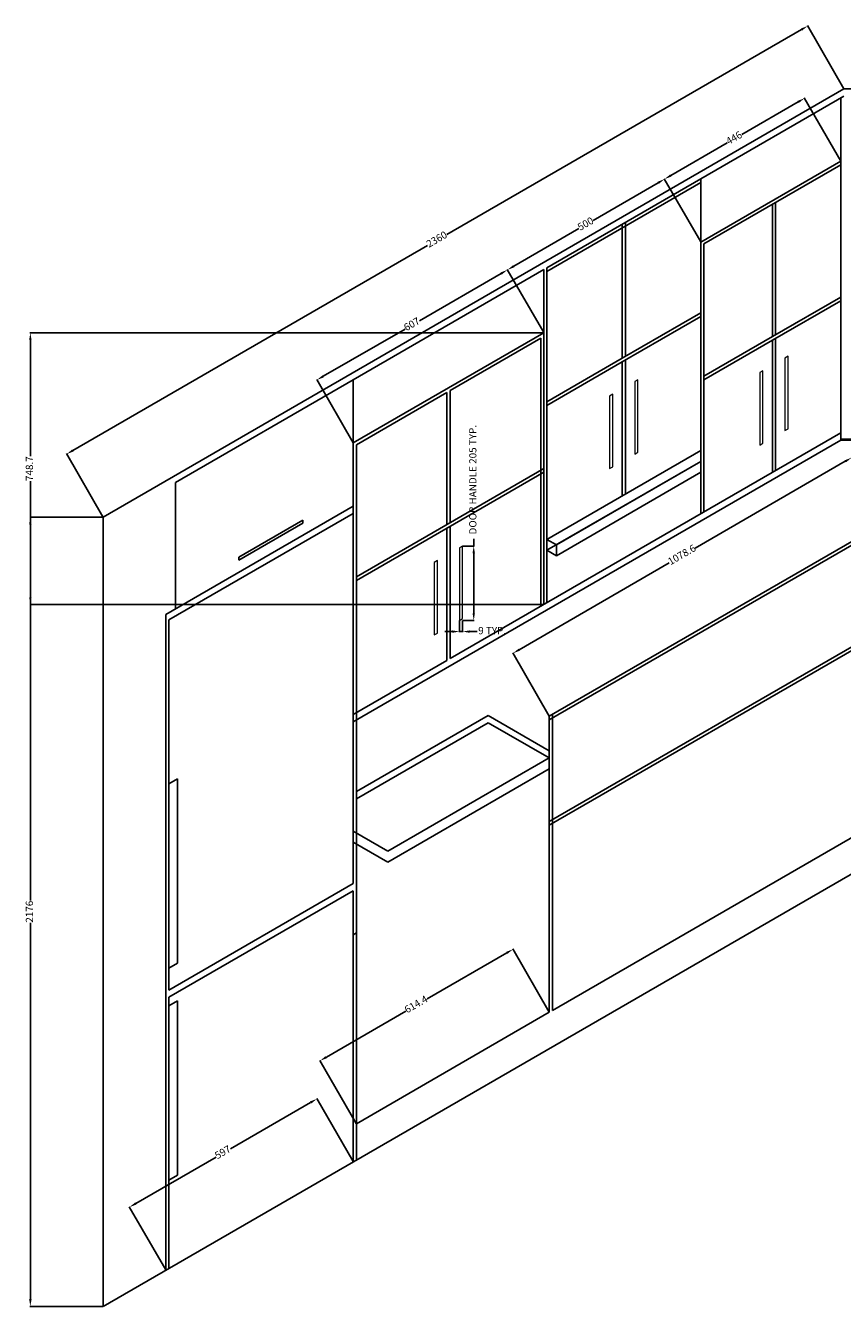
# Model space of a CAD drawing. Units: millimetres. Extents: x 78378 to 86415, y 148682 to 152721.
# Tile 17 of 18: x 82091 to 84344, y 149152 to 152682. Entities that reach past the tile are written whole.
import ezdxf

# ---------------------------------------------------------------- set-up
doc = ezdxf.new("R2010")
doc.units = ezdxf.units.MM
for name, color, linetype, lineweight in [('A-ANNO-DIMS', 2, 'Continuous', 18), ('A-FURN', 4, 'Continuous', 25), ('A-FURN-HRDW', 8, 'Continuous', 18)]:
    doc.layers.add(name, color=color, linetype=linetype, lineweight=lineweight)
doc.styles.get("Standard").update_dxf_attribs({"font": 'arial.ttf'})
doc.dimstyles.new('ISO-25', dxfattribs={"dimtxt": 20, "dimasz": 20, "dimexe": 1.25, "dimexo": 0.625, "dimtad": 0, "dimdec": 1, "dimtxsty": 'Standard', "dimcen": 2.5, "dimadec": 0, "dimazin": 0, "dimtfac": 1, "dimtdec": 1, "dimtmove": 0, "dimatfit": 3, "dimfxl": 1, "dimarcsym": 0})

# ---------------------------------------------------------------- blocks, each defined once
blk = doc.blocks.new('HANDLE-DOOR')
for p, q in [((8.7, 205), (0, 200)), ((0, 200), (0, 0)), ((8.7, 5), (8.7, 205)), ((0, 0), (8.7, 5))]:
    blk.add_line(p, q)
blk = doc.blocks.new('*D10')
at = {"layer": 'A-ANNO-DIMS', "color": 0, "lineweight": -2, "transparency": 16777216}
for p, q in [((83326.8, 151247.7), (83326.8, 151267.7)), ((83296.7, 151247.7), (83328, 151247.7)), ((83326.8, 151062.7), (83326.8, 151227.7)), ((83296.7, 151042.7), (83328, 151042.7))]:
    blk.add_line(p, q, dxfattribs=at)
at = {"layer": 'A-ANNO-DIMS', "color": 0, "transparency": 16777216}
for points in [[(83323.4, 151227.7), (83330.1, 151227.7), (83326.8, 151247.7)], [(83323.4, 151062.7), (83330.1, 151062.7), (83326.8, 151042.7)]]:
    blk.add_solid(points, dxfattribs=at)
at = {"layer": 'Defpoints', "color": 0, "transparency": 16777216}
for p in [(83296, 151247.7), (83326.8, 151247.7), (83296, 151042.7)]:
    blk.add_point(p, dxfattribs=at)
at = {"layer": 'A-ANNO-DIMS', "color": 0, "transparency": 16777216, "insert": (83326.8, 151430.6), "char_height": 20, "attachment_point": 5, "rotation": 90}
blk.add_mtext('DOOR HANDLE 205 TYP.', dxfattribs=at)
blk = doc.blocks.new('*D11')
at = {"layer": 'A-ANNO-DIMS', "color": 0, "lineweight": -2, "transparency": 16777216}
for p, q in [((83267.4, 151012), (83247.4, 151012)), ((83287.4, 151042.1), (83287.4, 151010.7)), ((83287.4, 151012), (83296, 151012)), ((83296, 151042.1), (83296, 151010.7)), ((83316, 151012), (83336, 151012))]:
    blk.add_line(p, q, dxfattribs=at)
at = {"layer": 'A-ANNO-DIMS', "color": 0, "transparency": 16777216}
for points in [[(83267.4, 151015.3), (83267.4, 151008.6), (83287.4, 151012)], [(83316, 151015.3), (83316, 151008.6), (83296, 151012)]]:
    blk.add_solid(points, dxfattribs=at)
at = {"layer": 'Defpoints', "color": 0, "transparency": 16777216}
for p in [(83287.4, 151042.7), (83296, 151042.7), (83296, 151012)]:
    blk.add_point(p, dxfattribs=at)
at = {"layer": 'A-ANNO-DIMS', "color": 0, "transparency": 16777216, "insert": (83377.6, 151012), "char_height": 20, "attachment_point": 5}
blk.add_mtext('9 TYP.', dxfattribs=at)
blk = doc.blocks.new('*D34')
at = {"layer": 'A-ANNO-DIMS', "color": 0, "lineweight": -2, "transparency": 16777216}
for p, q in [((82303.6, 151327.7), (82102.5, 151327.7)), ((82103.7, 151307.7), (82103.7, 150270.3)), ((82103.7, 149171.7), (82103.7, 150209)), ((82303.6, 149151.7), (82102.5, 149151.7))]:
    blk.add_line(p, q, dxfattribs=at)
at = {"layer": 'A-ANNO-DIMS', "color": 0, "transparency": 16777216}
for points in [[(82100.4, 151307.7), (82107.1, 151307.7), (82103.7, 151327.7)], [(82100.4, 149171.7), (82107.1, 149171.7), (82103.7, 149151.7)]]:
    blk.add_solid(points, dxfattribs=at)
at = {"layer": 'Defpoints', "color": 0, "transparency": 16777216}
for p in [(82103.7, 151327.7), (82304.2, 151327.7), (82304.2, 149151.7)]:
    blk.add_point(p, dxfattribs=at)
at = {"layer": 'A-ANNO-DIMS', "color": 0, "transparency": 16777216, "insert": (82103.7, 150239.7), "char_height": 20, "attachment_point": 5, "rotation": 90}
blk.add_mtext('2176', dxfattribs=at)
blk = doc.blocks.new('*D35')
at = {"layer": 'A-ANNO-DIMS', "color": 0, "lineweight": -2, "transparency": 16777216}
for p, q in [((84230.5, 152671.3), (83252.4, 152106.6)), ((84347.7, 152508.2), (84247.2, 152682.4)), ((82221.3, 151511.3), (83199.4, 152076)), ((82303.9, 151328.2), (82203.4, 151502.4))]:
    blk.add_line(p, q, dxfattribs=at)
at = {"layer": 'A-ANNO-DIMS', "color": 0, "transparency": 16777216}
for points in [[(84228.8, 152674.2), (84232.2, 152668.4), (84247.8, 152681.3)], [(82219.6, 151514.2), (82223, 151508.4), (82204, 151501.3)]]:
    blk.add_solid(points, dxfattribs=at)
at = {"layer": 'Defpoints', "color": 0, "transparency": 16777216}
for p in [(84247.8, 152681.3), (84348.1, 152507.7), (82304.2, 151327.7)]:
    blk.add_point(p, dxfattribs=at)
at = {"layer": 'A-ANNO-DIMS', "color": 0, "transparency": 16777216, "insert": (83225.9, 152091.3), "char_height": 20, "attachment_point": 5, "rotation": 30}
blk.add_mtext('2360', dxfattribs=at)
blk = doc.blocks.new('*D38')
at = {"layer": 'A-ANNO-DIMS', "color": 0, "lineweight": -2, "transparency": 16777216}
for p, q in [((84348.7, 152507.7), (86403.1, 152507.7)), ((86401.9, 152487.7), (86401.9, 152046.5)), ((86401.9, 151559.8), (86401.9, 152001)), ((84340, 151539.8), (86403.1, 151539.8))]:
    blk.add_line(p, q, dxfattribs=at)
at = {"layer": 'A-ANNO-DIMS', "color": 0, "transparency": 16777216}
for points in [[(86398.5, 152487.7), (86405.2, 152487.7), (86401.9, 152507.7)], [(86398.5, 151559.8), (86405.2, 151559.8), (86401.9, 151539.8)]]:
    blk.add_solid(points, dxfattribs=at)
at = {"layer": 'Defpoints', "color": 0, "transparency": 16777216}
for p in [(84348.1, 152507.7), (86401.9, 152507.7), (84339.4, 151539.8)]:
    blk.add_point(p, dxfattribs=at)
at = {"layer": 'A-ANNO-DIMS', "color": 0, "transparency": 16777216, "insert": (86401.9, 152023.7), "char_height": 20, "attachment_point": 5, "rotation": 90}
blk.add_mtext('968', dxfattribs=at)
blk = doc.blocks.new('*D39')
at = {"layer": 'A-ANNO-DIMS', "color": 0, "lineweight": -2, "transparency": 16777216}
for p, q in [((82876.9, 149713.8), (82655.4, 149585.9)), ((82994.2, 149550.7), (82893.6, 149724.9)), ((82394.5, 149435.3), (82616, 149563.2)), ((82477.1, 149252.2), (82376.6, 149426.4))]:
    blk.add_line(p, q, dxfattribs=at)
at = {"layer": 'A-ANNO-DIMS', "color": 0, "transparency": 16777216}
for points in [[(82875.2, 149716.7), (82878.6, 149710.9), (82894.2, 149723.8)], [(82392.9, 149438.2), (82396.2, 149432.4), (82377.2, 149425.3)]]:
    blk.add_solid(points, dxfattribs=at)
at = {"layer": 'Defpoints', "color": 0, "transparency": 16777216}
for p in [(82894.2, 149723.8), (82994.5, 149550.2), (82477.4, 149251.7)]:
    blk.add_point(p, dxfattribs=at)
at = {"layer": 'A-ANNO-DIMS', "color": 0, "transparency": 16777216, "insert": (82635.7, 149574.6), "char_height": 20, "attachment_point": 5, "rotation": 30}
blk.add_mtext('597', dxfattribs=at)
blk = doc.blocks.new('*D40')
at = {"layer": 'A-ANNO-DIMS', "color": 0, "lineweight": -2, "transparency": 16777216}
for p, q in [((83534.9, 149962.9), (83434.4, 150137.1)), ((83417.7, 150126), (83198.7, 149999.6)), ((82920.2, 149838.8), (83139.2, 149965.2)), ((83002.8, 149655.7), (82902.2, 149829.9))]:
    blk.add_line(p, q, dxfattribs=at)
at = {"layer": 'A-ANNO-DIMS', "color": 0, "transparency": 16777216}
for points in [[(83416, 150128.9), (83419.3, 150123.2), (83435, 150136)], [(82918.5, 149841.7), (82921.9, 149835.9), (82902.9, 149828.8)]]:
    blk.add_solid(points, dxfattribs=at)
at = {"layer": 'Defpoints', "color": 0, "transparency": 16777216}
for p in [(83435, 150136), (83535.2, 149962.4), (83003.1, 149655.2)]:
    blk.add_point(p, dxfattribs=at)
at = {"layer": 'A-ANNO-DIMS', "color": 0, "transparency": 16777216, "insert": (83168.9, 149982.4), "char_height": 20, "attachment_point": 5, "rotation": 30}
blk.add_mtext('614.4', dxfattribs=at)
blk = doc.blocks.new('*D41')
at = {"layer": 'A-ANNO-DIMS', "color": 0, "lineweight": -2, "transparency": 16777216}
for p, q in [((84351.7, 151481.3), (83937.7, 151242.3)), ((84469, 151318.2), (84368.4, 151492.4)), ((83452.3, 150962), (83866.3, 151201.1)), ((83534.9, 150778.9), (83434.4, 150953.1))]:
    blk.add_line(p, q, dxfattribs=at)
at = {"layer": 'A-ANNO-DIMS', "color": 0, "transparency": 16777216}
for points in [[(84350.1, 151484.2), (84353.4, 151478.4), (84369.1, 151491.3)], [(83450.6, 150964.9), (83454, 150959.2), (83435, 150952)]]:
    blk.add_solid(points, dxfattribs=at)
at = {"layer": 'Defpoints', "color": 0, "transparency": 16777216}
for p in [(84369.1, 151491.3), (84469.3, 151317.7), (83535.2, 150778.4)]:
    blk.add_point(p, dxfattribs=at)
at = {"layer": 'A-ANNO-DIMS', "color": 0, "transparency": 16777216, "insert": (83902, 151221.7), "char_height": 20, "attachment_point": 5, "rotation": 30}
blk.add_mtext('1078.6', dxfattribs=at)
blk = doc.blocks.new('*D42')
at = {"layer": 'A-ANNO-DIMS', "color": 0, "lineweight": -2, "transparency": 16777216}
for p, q in [((83402.6, 151999.1), (83176.8, 151868.7)), ((83519.8, 151836), (83419.3, 152010.2)), ((82911.5, 151715.6), (83137.3, 151846)), ((82994.2, 151532.5), (82893.6, 151706.7))]:
    blk.add_line(p, q, dxfattribs=at)
at = {"layer": 'A-ANNO-DIMS', "color": 0, "transparency": 16777216}
for points in [[(83400.9, 152002), (83404.2, 151996.2), (83419.9, 152009.1)], [(82909.9, 151718.5), (82913.2, 151712.7), (82894.2, 151705.6)]]:
    blk.add_solid(points, dxfattribs=at)
at = {"layer": 'Defpoints', "color": 0, "transparency": 16777216}
for p in [(83419.9, 152009.1), (83520.1, 151835.5), (82994.5, 151532)]:
    blk.add_point(p, dxfattribs=at)
at = {"layer": 'A-ANNO-DIMS', "color": 0, "transparency": 16777216, "insert": (83157.1, 151857.3), "char_height": 20, "attachment_point": 5, "rotation": 30}
blk.add_mtext('607', dxfattribs=at)
blk = doc.blocks.new('*D43')
at = {"layer": 'A-ANNO-DIMS', "color": 0, "lineweight": -2, "transparency": 16777216}
for p, q in [((83835.6, 152249.1), (83656, 152145.4)), ((83952.8, 152086), (83852.3, 152260.2)), ((83437.2, 152019.1), (83616.8, 152122.8)), ((83519.8, 151836), (83419.3, 152010.2))]:
    blk.add_line(p, q, dxfattribs=at)
at = {"layer": 'A-ANNO-DIMS', "color": 0, "transparency": 16777216}
for points in [[(83833.9, 152252), (83837.3, 152246.2), (83852.9, 152259.1)], [(83435.5, 152022), (83438.9, 152016.2), (83419.9, 152009.1)]]:
    blk.add_solid(points, dxfattribs=at)
at = {"layer": 'Defpoints', "color": 0, "transparency": 16777216}
for p in [(83852.9, 152259.1), (83953.2, 152085.5), (83520.1, 151835.5)]:
    blk.add_point(p, dxfattribs=at)
at = {"layer": 'A-ANNO-DIMS', "color": 0, "transparency": 16777216, "insert": (83636.4, 152134.1), "char_height": 20, "attachment_point": 5, "rotation": 30}
blk.add_mtext('500', dxfattribs=at)
blk = doc.blocks.new('*D44')
at = {"layer": 'A-ANNO-DIMS', "color": 0, "lineweight": -2, "transparency": 16777216}
for p, q in [((84221.8, 152472.1), (84066, 152382.2)), ((84339.1, 152309), (84238.5, 152483.2)), ((83870.2, 152269.1), (84026, 152359)), ((83952.8, 152086), (83852.3, 152260.2))]:
    blk.add_line(p, q, dxfattribs=at)
at = {"layer": 'A-ANNO-DIMS', "color": 0, "transparency": 16777216}
for points in [[(84220.2, 152475), (84223.5, 152469.2), (84239.2, 152482.1)], [(83868.6, 152272), (83871.9, 152266.2), (83852.9, 152259.1)]]:
    blk.add_solid(points, dxfattribs=at)
at = {"layer": 'Defpoints', "color": 0, "transparency": 16777216}
for p in [(84239.2, 152482.1), (84339.4, 152308.5), (83953.2, 152085.5)]:
    blk.add_point(p, dxfattribs=at)
at = {"layer": 'A-ANNO-DIMS', "color": 0, "transparency": 16777216, "insert": (84046, 152370.6), "char_height": 20, "attachment_point": 5, "rotation": 30}
blk.add_mtext('446', dxfattribs=at)
blk = doc.blocks.new('*D45')
at = {"layer": 'A-ANNO-DIMS', "color": 0, "lineweight": -2, "transparency": 16777216}
for p, q in [((83519.5, 151835.5), (82102.5, 151835.5)), ((82103.7, 151815.5), (82103.7, 151495.4)), ((82103.7, 151106.8), (82103.7, 151426.8)), ((83519.5, 151086.8), (82102.5, 151086.8))]:
    blk.add_line(p, q, dxfattribs=at)
at = {"layer": 'A-ANNO-DIMS', "color": 0, "transparency": 16777216}
for points in [[(82100.4, 151815.5), (82107.1, 151815.5), (82103.7, 151835.5)], [(82100.4, 151106.8), (82107.1, 151106.8), (82103.7, 151086.8)]]:
    blk.add_solid(points, dxfattribs=at)
at = {"layer": 'Defpoints', "color": 0, "transparency": 16777216}
for p in [(82103.7, 151835.5), (83520.1, 151835.5), (83520.1, 151086.8)]:
    blk.add_point(p, dxfattribs=at)
at = {"layer": 'A-ANNO-DIMS', "color": 0, "transparency": 16777216, "insert": (82103.7, 151461.1), "char_height": 20, "attachment_point": 5, "rotation": 90}
blk.add_mtext('748.7', dxfattribs=at)

msp = doc.modelspace()

# ---------------------------------------------------------------- linework, layer by layer
at = {"layer": 'A-FURN'}
for p, q in [((82304.2424, 151327.6946), (84348.0623, 152507.6946)), ((83953.1548, 152259.6946), (84348.0623, 152487.6946)), ((84339.4021, 152482.6946), (84339.4021, 151539.7603)), ((83953.1548, 152085.457), (84339.4021, 152308.457)), ((83961.815, 152080.457), (84339.4021, 152298.457)), ((84339.4021, 152298.457), (84339.4021, 151539.7603)), ((83528.8023, 152014.6946), (83953.1548, 152259.6946)), ((83528.8023, 152004.6946), (83953.1548, 152249.6946)), ((83953.1548, 151336.7603), (83953.1548, 152259.6946)), ((84150.6086, 152189.457), (84150.6086, 151825.1086)), ((84159.2688, 152194.457), (84159.2688, 151830.1086)), ((83745.3087, 152139.6946), (83745.3087, 151770.3463)), ((83736.6484, 152134.6946), (83736.6484, 151765.3463)), ((83961.815, 151341.7603), (83961.815, 152080.457)), ((82994.4646, 151706.1946), (83520.1421, 152009.6946)), ((83520.1421, 151086.7603), (83520.1421, 152009.6946)), ((83528.8023, 151091.7603), (83528.8023, 152014.6946)), ((84150.6086, 151825.1086), (84339.4021, 151934.1086)), ((84150.6086, 151815.1086), (84339.4021, 151924.1086)), ((83736.6484, 151765.3463), (83953.1548, 151890.3463)), ((83736.6484, 151755.3463), (83953.1548, 151880.3463)), ((82994.4646, 151531.957), (83520.1421, 151835.457)), ((83961.815, 151716.1086), (84150.6086, 151825.1086)), ((83261.6335, 151676.207), (83511.4818, 151820.457)), ((83511.4818, 151081.7603), (83511.4818, 151820.457)), ((83961.815, 151706.1086), (84150.6086, 151815.1086)), ((84150.6086, 151815.1086), (84150.6086, 151450.7603)), ((84159.2688, 151820.1086), (84159.2688, 151455.7603)), ((83528.8023, 151645.3463), (83736.6484, 151765.3463)), ((83528.8023, 151635.3463), (83736.6484, 151755.3463)), ((83736.6484, 151755.3463), (83736.6484, 151385.9979)), ((83745.3087, 151760.3463), (83745.3087, 151390.9979)), ((82503.8506, 151422.9385), (82994.4646, 151706.1946)), ((82994.4646, 150317.1892), (82994.4646, 151706.1946)), ((83003.1249, 151526.957), (83252.9732, 151671.207)), ((83252.9732, 151671.207), (83252.9732, 151306.8586)), ((83261.6335, 151676.207), (83261.6335, 151311.8586)), ((84339.4021, 151539.7603), (82994.4646, 150763.2603)), ((84339.4021, 151559.7603), (83261.6335, 150937.5103)), ((84599.2097, 151542.6946), (84339.4021, 151542.6946)), ((83003.1249, 149555.1946), (83003.1249, 151526.957)), ((83528.8023, 151265.9979), (83953.1548, 151510.9979)), ((83528.8023, 151235.9979), (83953.1548, 151480.9979)), ((83554.7831, 151250.9979), (83953.1548, 151480.9979)), ((83520.1421, 151461.1086), (83003.1249, 151162.6086)), ((83520.1421, 151451.1086), (83003.1249, 151152.6086)), ((83554.7831, 151220.9979), (83953.1548, 151450.9979)), ((82503.8506, 151422.9385), (82503.8506, 151074.4631)), ((82304.2424, 149151.6946), (82304.2424, 151327.6946)), ((82477.4475, 151059.2193), (82994.4646, 151357.7193)), ((82486.1077, 151044.2193), (82994.4646, 151337.7193)), ((82855.7689, 151319.1676), (82679.0417, 151217.1342)), ((82679.0417, 151208.5443), (82855.7689, 151310.5778)), ((82855.7689, 151310.5778), (82855.7689, 151319.1676)), ((83252.9732, 151296.8586), (83252.9732, 150932.5103)), ((83261.6335, 151301.8586), (83261.6335, 150937.5103)), ((84469.3059, 151317.6946), (83535.2323, 150778.407)), ((84477.9662, 151312.6946), (83535.2323, 150768.407)), ((83528.8023, 151265.9979), (83528.8023, 151235.9979)), ((83528.8023, 151265.9979), (83554.7831, 151250.9979)), ((83528.8023, 151235.9979), (83554.7831, 151220.9979)), ((83554.7831, 151250.9979), (83554.7831, 151220.9979)), ((82679.0417, 151208.5443), (82679.0417, 151217.1342)), ((84720.4533, 151172.6946), (83535.2323, 150488.407)), ((82477.4475, 149251.6946), (82477.4475, 151059.2193)), ((82486.1077, 150023.6892), (82486.1077, 151044.2193)), ((84469.3059, 151017.6946), (83535.2323, 150478.407)), ((83252.9732, 150932.5103), (82994.4646, 150783.2603)), ((83003.1249, 150570.6888), (83366.9976, 150780.7708)), ((83535.2323, 150683.6404), (83366.9976, 150780.7708)), ((83535.2323, 150778.407), (83535.2323, 149962.407)), ((83543.8926, 150783.407), (83543.8926, 149967.407)), ((83003.1249, 150550.6888), (83366.9976, 150760.7708)), ((83535.2323, 150663.6404), (83366.9976, 150760.7708)), ((83089.7274, 150406.428), (83535.2323, 150663.6404)), ((83089.7274, 150376.428), (83535.2323, 150633.6404)), ((82509.649, 150606.068), (82486.1077, 150592.4765)), ((82509.649, 150097.4215), (82509.649, 150606.068)), ((83543.8926, 149967.407), (84469.3059, 150501.6946)), ((83089.7274, 150406.428), (82994.4646, 150461.428)), ((83089.7274, 150376.428), (82994.4646, 150431.428)), ((82304.2424, 149151.6946), (84469.3059, 150401.6946)), ((82486.1077, 150023.6892), (82994.4646, 150317.1892)), ((82486.1077, 150003.6892), (82994.4646, 150297.1892)), ((82994.4646, 149550.1946), (82994.4646, 150297.1892)), ((83003.1249, 150181.1946), (82994.4646, 150176.1946)), ((82509.649, 150097.4215), (82486.1077, 150083.83)), ((82486.1077, 149256.6946), (82486.1077, 150003.6892)), ((82486.1077, 149980.5031), (82509.649, 149994.0946)), ((82509.649, 149994.0946), (82509.649, 149513.5558)), ((83003.1249, 149655.1946), (83535.2323, 149962.407)), ((82509.649, 149513.5558), (82486.1077, 149499.9643))]:
    msp.add_line(p, q, dxfattribs=at)

# ---------------------------------------------------------------- block references
at = {"layer": 'A-FURN-HRDW'}
for p in [(84185.184, 151566.0597), (84115.8717, 151526.0423), (83771.0442, 151501.1937), (83701.7319, 151461.1762), (83287.369, 151042.706), (83218.0567, 151002.6885)]:
    msp.add_blockref('HANDLE-DOOR', p, dxfattribs=at)

# ---------------------------------------------------------------- dimensions: what is measured, and where the dimension line sits
at = {"layer": 'A-ANNO-DIMS'}
for base, p1, p2, angle, override, picture, middle in [((84247.8123, 152681.3327), (82304.2424, 151327.6946), (84348.0623, 152507.6946), 30, {"dimdec": 0, "dimlfac": 1, "dimrnd": 0, "dimzin": 0, "dimdsep": 46, "dimlunit": 2}, '*D35', (83225.9024, 152091.3327)), ((86401.8567, 152507.6946), (84339.4021, 151539.7603), (84348.0623, 152507.6946), 90, {"dimdec": 0, "dimlfac": 1, "dimrnd": 0, "dimzin": 0, "dimdsep": 46, "dimlunit": 2}, '*D38', (86401.8567, 152023.7274)), ((84239.1521, 152482.095), (83953.1548, 152085.457), (84339.4021, 152308.457), 30, {"dimdec": 0, "dimlfac": 1, "dimrnd": 0, "dimzin": 0, "dimdsep": 46, "dimlunit": 2}, '*D44', (84046.0284, 152370.595)), ((83852.9048, 152259.095), (83520.1421, 151835.457), (83953.1548, 152085.457), 30, {"dimdec": 0, "dimlfac": 1, "dimrnd": 0, "dimzin": 0, "dimdsep": 46, "dimlunit": 2}, '*D43', (83636.3984, 152134.095)), ((83419.8921, 152009.095), (82994.4646, 151531.957), (83520.1421, 151835.457), 30, {"dimdec": 0, "dimlfac": 1, "dimrnd": 0, "dimzin": 0, "dimdsep": 46, "dimlunit": 2}, '*D42', (83157.0534, 151857.345)), ((82103.7424, 151835.457), (83520.1421, 151086.7603), (83520.1421, 151835.457), 90, {"dimdec": 1, "dimlfac": 1, "dimrnd": 0, "dimzin": 0, "dimdsep": 46, "dimlunit": 2}, '*D45', (82103.7424, 151461.1086)), ((84369.0559, 151491.3327), (83535.2323, 150778.407), (84469.3059, 151317.6946), 30, {"dimdec": 1, "dimlfac": 1, "dimrnd": 0, "dimzin": 0, "dimdsep": 46, "dimlunit": 2}, '*D41', (83902.0191, 151221.6889)), ((82103.7424, 151327.6946), (82304.2424, 149151.6946), (82304.2424, 151327.6946), 90, {"dimdec": 0, "dimlfac": 1, "dimrnd": 0, "dimzin": 0, "dimdsep": 46, "dimlunit": 2}, '*D34', (82103.7424, 150239.6946)), ((83434.9823, 150136.0451), (83003.1249, 149655.1946), (83535.2323, 149962.407), 30, {"dimdec": 1, "dimlfac": 1, "dimrnd": 0, "dimzin": 0, "dimdsep": 46, "dimlunit": 2}, '*D40', (83168.9286, 149982.4389)), ((82894.2146, 149723.8327), (82477.4475, 149251.6946), (82994.4646, 149550.1946), 30, {"dimdec": 0, "dimlfac": 1, "dimrnd": 0, "dimzin": 0, "dimdsep": 46, "dimlunit": 2}, '*D39', (82635.7061, 149574.5827))]:
    dim = msp.add_linear_dim(base=base, p1=p1, p2=p2, angle=angle, dimstyle='ISO-25', override=override, dxfattribs=at)
    dim.commit()
    dim.dimension.update_dxf_attribs({"geometry": picture, "text_midpoint": middle})
dim = msp.add_linear_dim(base=(83326.7792, 151247.7056), p1=(83296.0292, 151042.7056), p2=(83296.0292, 151247.7056), angle=90, text='DOOR HANDLE <> TYP.', dimstyle='ISO-25', override={"dimdec": 0, "dimrnd": 0, "dimzin": 0, "dimlunit": 2}, dxfattribs=at)
dim.commit()
dim.dimension.update_dxf_attribs({"geometry": '*D10', "text_midpoint": (83326.7792, 151430.6226)})
dim = msp.add_linear_dim(base=(83296.0292, 151011.9556), p1=(83287.3689, 151042.7056), p2=(83296.0292, 151042.7056), text='<> TYP.', dimstyle='ISO-25', override={"dimdec": 0, "dimrnd": 0, "dimzin": 0, "dimlunit": 2}, dxfattribs=at)
dim.commit()
dim.dimension.update_dxf_attribs({"geometry": '*D11', "text_midpoint": (83377.5614, 151011.9556)})

doc.saveas('drawing.dxf')
